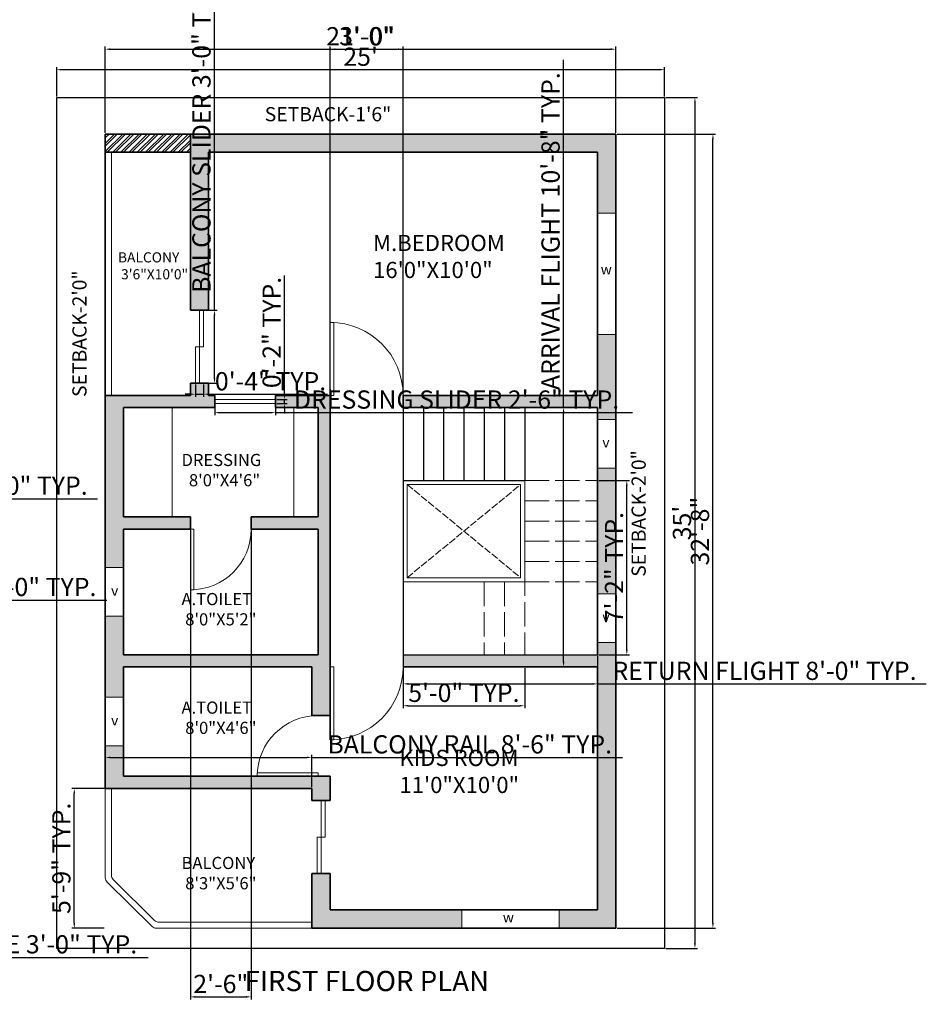
# Model space of a CAD drawing. Units: inches. Extents: x 3488 to 4319, y 780 to 1756.
# Tile 2 of 8: x 3872 to 4319, y 788 to 1274. Entities that reach past the tile are written whole.
import ezdxf

# ---------------------------------------------------------------- set-up
doc = ezdxf.new("R2010")
doc.units = ezdxf.units.IN
doc.linetypes.add('ACAD_ISO02W100', pattern=[15, 12, -3])
for name, color, linetype, lineweight in [('A-ANNO-IDEN', 7, 'Continuous', 13), ('A-ANNO-TEXT', 7, 'Continuous', 18), ('A-ANNO-TITL', 7, 'Continuous', 25), ('A-AREA-IDEN', 7, 'Continuous', 18), ('A-DOOR', 4, 'Continuous', 18), ('A-FLOR-CASE', 32, 'Continuous', 18), ('A-FLOR-OPEN', 3, 'Continuous', 20), ('A-FLOR-OPEN-HIDN', 3, 'ACAD_ISO02W100', 13), ('A-FLOR-RAIL', 7, 'Continuous', 20), ('A-FLOR-STRS', 7, 'Continuous', 25), ('A-FLOR-STRS-OVHD', 8, 'ACAD_ISO02W100', 18), ('A-WALL', 7, 'Continuous', 35), ('A-WALL-PATT', 252, 'Continuous', 13), ('C-PROP', 7, 'Continuous', 25), ('DIM', 9, 'Continuous', 18), ('window', 130, 'Continuous', 18)]:
    doc.layers.add(name, color=color, linetype=linetype, lineweight=lineweight)
doc.styles.get("Standard").update_dxf_attribs({"font": 'arial.ttf'})
doc.dimstyles.new('ISO-25', dxfattribs={"dimtxt": 9, "dimasz": 2.5, "dimexe": 1.25, "dimexo": 0.625, "dimtad": 1, "dimdec": 1, "dimlunit": 3, "dimtxsty": 'Standard', "dimcen": 2.5, "dimclrd": 1, "dimclre": 1, "dimclrt": 1, "dimadec": 0, "dimazin": 0, "dimtfac": 1, "dimtdec": 1, "dimtmove": 0, "dimatfit": 3, "dimfxl": 1, "dimarcsym": 0})

# ---------------------------------------------------------------- blocks, each defined once
blk = doc.blocks.new('*U3')
for p, q in [((0, 0), (0, -6)), ((36, 0), (36, -6))]:
    blk.add_line(p, q)
blk.add_lwpolyline([(0, 0), (0, 36), (1.75, 36), (1.75, 0)], close=True)
blk.add_arc((0, 0), 36, 0, 90)
blk = doc.blocks.new('*D13')
at = {"layer": 'Defpoints', "color": 0, "transparency": 16777216}
for p in [(4189.84, 1249.81), (3889.84, 1236.01), (4189.84, 1236.01)]:
    blk.add_point(p, dxfattribs=at)
at = {"layer": 'DIM', "color": 0, "lineweight": -2, "transparency": 16777216}
for p, q in [((3889.84, 1236.63), (3889.84, 1251.06)), ((3892.34, 1249.81), (4187.34, 1249.81)), ((4189.84, 1236.63), (4189.84, 1251.06))]:
    blk.add_line(p, q, dxfattribs=at)
at = {"layer": 'DIM', "color": 0, "transparency": 16777216}
for points in [[(3892.34, 1250.23), (3892.34, 1249.39), (3889.84, 1249.81)], [(4187.34, 1250.23), (4187.34, 1249.39), (4189.84, 1249.81)]]:
    blk.add_solid(points, dxfattribs=at)
at = {"layer": 'DIM', "color": 0, "transparency": 16777216, "insert": (4039.84, 1255.03), "char_height": 9, "attachment_point": 5}
blk.add_mtext("25'", dxfattribs=at)
blk = doc.blocks.new('*D12')
at = {"layer": 'Defpoints', "color": 0, "transparency": 16777216}
for p in [(4189.84, 1236.01), (4189.84, 816.01), (4204.87, 816.01)]:
    blk.add_point(p, dxfattribs=at)
at = {"layer": 'DIM', "color": 0, "lineweight": -2, "transparency": 16777216}
for p, q in [((4190.47, 1236.01), (4206.12, 1236.01)), ((4204.87, 1233.51), (4204.87, 818.51)), ((4190.47, 816.01), (4206.12, 816.01))]:
    blk.add_line(p, q, dxfattribs=at)
at = {"layer": 'DIM', "color": 0, "transparency": 16777216}
for points in [[(4204.45, 1233.51), (4205.28, 1233.51), (4204.87, 1236.01)], [(4204.45, 818.51), (4205.28, 818.51), (4204.87, 816.01)]]:
    blk.add_solid(points, dxfattribs=at)
at = {"layer": 'DIM', "color": 0, "transparency": 16777216, "insert": (4199.64, 1026.01), "char_height": 9, "attachment_point": 5, "rotation": 90}
blk.add_mtext("35'", dxfattribs=at)
blk = doc.blocks.new('*U9')
for p, q in [((0, 0), (0, 6)), ((36, 0), (36, 6))]:
    blk.add_line(p, q)
blk.add_lwpolyline([(0, 0), (0, -36), (1.75, -36), (1.75, 0)], close=True)
blk.add_arc((0, 0), 36, 270, 0)
blk = doc.blocks.new('*U10')
for p, q in [((0, 0), (0, 6)), ((30, 0), (30, 6))]:
    blk.add_line(p, q)
blk.add_lwpolyline([(0, 0), (0, -30), (1.75, -30), (1.75, 0)], close=True)
blk.add_arc((0, 0), 30, 270, 0)
blk = doc.blocks.new('*U11')
for p, q in [((-30, 0), (-30, 6)), ((0, 0), (0, 6))]:
    blk.add_line(p, q)
blk.add_lwpolyline([(0, 0), (0, -30), (-1.75, -30), (-1.75, 0)], close=True)
blk.add_arc((0, 0), 30, 180, 270)
blk = doc.blocks.new('DOOR-SLIDING-36IN')
for p, q in [((2, 0), (2, 36)), ((4, 18), (4, 36)), ((0, 0), (0, 18)), ((0, 18), (4, 18))]:
    blk.add_line(p, q)
blk = doc.blocks.new('RAIL-BALCONY-CHAMFERED')
for p, q in [((0, 69), (0, 24.92)), ((3, 69), (3, 26.17)), ((23.12, 0.86), (0.89, 22.78)), ((24.35, 3.86), (3.89, 24.04)), ((102, 3), (26.46, 3)), ((102, 0), (25.23, 0))]:
    blk.add_line(p, q)
for centre, start, end in [((3, 24.92), 180, 225.4044), ((6, 26.17), 180, 225.4044), ((25.23, 3), 225.4044, 270), ((26.46, 6), 225.4044, 270)]:
    blk.add_arc(centre, 3, start, end)
blk = doc.blocks.new('STAIR-UPPER-RETURN-BEYOND')
for p, q in [((60, 86), (60, 0)), ((60, 86), (96, 86)), ((60, 76), (96, 76)), ((60, 66), (96, 66)), ((60, 56), (96, 56)), ((60, 46), (96, 46)), ((0, 36), (96, 36)), ((40, 36), (40, 0)), ((50, 36), (50, 0))]:
    blk.add_line(p, q)
blk = doc.blocks.new('STAIR-UPPER-ARRIVAL-FLIGHT')
for p, q in [((0, 128), (0, 0)), ((10, 128), (10, 92)), ((20, 128), (20, 92)), ((30, 128), (30, 92)), ((40, 128), (40, 92)), ((50, 128), (50, 92)), ((60, 128), (60, 92)), ((0, 92), (60, 92))]:
    blk.add_line(p, q)
blk = doc.blocks.new('OPENING-STAIRWELL-FRAME')
for points in [[(60, 50), (0, 50), (0, 0), (60, 0)], [(58, 48), (2, 48), (2, 2), (58, 2)]]:
    blk.add_lwpolyline(points, close=True)
blk = doc.blocks.new('DOOR-SLIDING-30IN')
for p, q in [((30, 2), (0, 2)), ((30, 0), (0, 0))]:
    blk.add_line(p, q)
blk = doc.blocks.new('*D58')
at = {"layer": 'Defpoints', "color": 0, "transparency": 16777216}
for p in [(3962.34, 1131.01), (3967.74, 1131.01), (3962.34, 1095.01)]:
    blk.add_point(p, dxfattribs=at)
at = {"layer": 'DIM', "color": 1, "lineweight": -2, "transparency": 16777216}
for p, q in [((3967.74, 1131.01), (3967.74, 1301.71)), ((3962.97, 1131.01), (3968.99, 1131.01)), ((3967.74, 1097.51), (3967.74, 1128.51)), ((3962.97, 1095.01), (3968.99, 1095.01))]:
    blk.add_line(p, q, dxfattribs=at)
at = {"layer": 'DIM', "color": 1, "transparency": 16777216}
for points in [[(3967.33, 1128.51), (3968.16, 1128.51), (3967.74, 1131.01)], [(3967.33, 1097.51), (3968.16, 1097.51), (3967.74, 1095.01)]]:
    blk.add_solid(points, dxfattribs=at)
at = {"layer": 'DIM', "color": 1, "transparency": 16777216, "insert": (3962.46, 1217.61), "char_height": 9, "attachment_point": 5, "rotation": 90}
blk.add_mtext('BALCONY SLIDER 3\'-0" TYP.', dxfattribs=at)
blk = doc.blocks.new('*D59')
at = {"layer": 'Defpoints', "color": 0, "transparency": 16777216}
for p in [(3958.34, 1095.01), (3962.34, 1095.01), (3962.34, 1089.61)]:
    blk.add_point(p, dxfattribs=at)
at = {"layer": 'DIM', "color": 1, "lineweight": -2, "transparency": 16777216}
for p, q in [((3958.34, 1094.38), (3958.34, 1088.36)), ((3962.34, 1094.38), (3962.34, 1088.36)), ((3955.84, 1089.61), (3953.34, 1089.61)), ((3958.34, 1089.61), (3962.34, 1089.61)), ((3964.84, 1089.61), (4023.45, 1089.61))]:
    blk.add_line(p, q, dxfattribs=at)
at = {"layer": 'DIM', "color": 1, "transparency": 16777216}
for points in [[(3955.84, 1090.02), (3955.84, 1089.19), (3958.34, 1089.61)], [(3964.84, 1090.02), (3964.84, 1089.19), (3962.34, 1089.61)]]:
    blk.add_solid(points, dxfattribs=at)
at = {"layer": 'DIM', "color": 1, "transparency": 16777216, "insert": (3995.4, 1094.83), "char_height": 9, "attachment_point": 5}
blk.add_mtext('0\'-4" TYP.', dxfattribs=at)
blk = doc.blocks.new('*D60')
at = {"layer": 'Defpoints', "color": 0, "transparency": 16777216}
for p in [(3693.99, 997.01), (3753.99, 997.01), (3753.99, 988.01)]:
    blk.add_point(p, dxfattribs=at)
at = {"layer": 'DIM', "color": 1, "lineweight": -2, "transparency": 16777216}
for p, q in [((3693.99, 996.38), (3693.99, 986.76)), ((3753.99, 996.38), (3753.99, 986.76)), ((3696.49, 988.01), (3751.49, 988.01)), ((3753.99, 988.01), (3914.55, 988.01))]:
    blk.add_line(p, q, dxfattribs=at)
at = {"layer": 'DIM', "color": 1, "transparency": 16777216}
for points in [[(3696.49, 988.42), (3696.49, 987.59), (3693.99, 988.01)], [(3751.49, 988.42), (3751.49, 987.59), (3753.99, 988.01)]]:
    blk.add_solid(points, dxfattribs=at)
at = {"layer": 'DIM', "color": 1, "transparency": 16777216, "insert": (3835.52, 993.29), "char_height": 9, "attachment_point": 5}
blk.add_mtext('STAIR OPENING 5\'-0" TYP.', dxfattribs=at)
blk = doc.blocks.new('*D70')
at = {"layer": 'Defpoints', "color": 0, "transparency": 16777216}
for p in [(3756.99, 817.01), (3792.99, 817.01), (3792.99, 811.61)]:
    blk.add_point(p, dxfattribs=at)
at = {"layer": 'DIM', "color": 1, "lineweight": -2, "transparency": 16777216}
for p, q in [((3756.99, 816.38), (3756.99, 810.36)), ((3792.99, 816.38), (3792.99, 810.36)), ((3759.49, 811.61), (3790.49, 811.61)), ((3792.99, 811.61), (3934.96, 811.61))]:
    blk.add_line(p, q, dxfattribs=at)
at = {"layer": 'DIM', "color": 1, "transparency": 16777216}
for points in [[(3759.49, 812.02), (3759.49, 811.19), (3756.99, 811.61)], [(3790.49, 812.02), (3790.49, 811.19), (3792.99, 811.61)]]:
    blk.add_solid(points, dxfattribs=at)
at = {"layer": 'DIM', "color": 1, "transparency": 16777216, "insert": (3865.22, 816.89), "char_height": 9, "attachment_point": 5}
blk.add_mtext('ENTRY GATE 3\'-0" TYP.', dxfattribs=at)
blk = doc.blocks.new('*D72')
at = {"layer": 'Defpoints', "color": 0, "transparency": 16777216}
for p in [(4015.84, 910.31), (3913.84, 895.01), (4015.84, 895.01)]:
    blk.add_point(p, dxfattribs=at)
at = {"layer": 'DIM', "color": 1, "lineweight": -2, "transparency": 16777216}
for p, q in [((3913.84, 895.63), (3913.84, 911.56)), ((3916.34, 910.31), (4013.34, 910.31)), ((4015.84, 895.63), (4015.84, 911.56)), ((4015.84, 910.31), (4169.08, 910.31))]:
    blk.add_line(p, q, dxfattribs=at)
at = {"layer": 'DIM', "color": 1, "transparency": 16777216}
for points in [[(3916.34, 910.72), (3916.34, 909.89), (3913.84, 910.31)], [(4013.34, 910.72), (4013.34, 909.89), (4015.84, 910.31)]]:
    blk.add_solid(points, dxfattribs=at)
at = {"layer": 'DIM', "color": 1, "transparency": 16777216, "insert": (4093.71, 915.59), "char_height": 9, "attachment_point": 5}
blk.add_mtext('BALCONY RAIL 8\'-6" TYP.', dxfattribs=at)
blk = doc.blocks.new('*D73')
at = {"layer": 'Defpoints', "color": 0, "transparency": 16777216}
for p in [(3898.54, 895.01), (3913.84, 895.01), (3913.84, 826.01)]:
    blk.add_point(p, dxfattribs=at)
at = {"layer": 'DIM', "color": 1, "lineweight": -2, "transparency": 16777216}
for p, q in [((3913.22, 895.01), (3897.29, 895.01)), ((3898.54, 828.51), (3898.54, 892.51)), ((3913.22, 826.01), (3897.29, 826.01))]:
    blk.add_line(p, q, dxfattribs=at)
at = {"layer": 'DIM', "color": 1, "transparency": 16777216}
for points in [[(3898.13, 892.51), (3898.96, 892.51), (3898.54, 895.01)], [(3898.13, 828.51), (3898.96, 828.51), (3898.54, 826.01)]]:
    blk.add_solid(points, dxfattribs=at)
at = {"layer": 'DIM', "color": 1, "transparency": 16777216, "insert": (3893.32, 860.51), "char_height": 9, "attachment_point": 5, "rotation": 90}
blk.add_mtext('5\'-9" TYP.', dxfattribs=at)
blk = doc.blocks.new('*D74')
at = {"layer": 'Defpoints', "color": 0, "transparency": 16777216}
for p in [(3693.99, 1047.01), (3753.99, 1047.01), (3753.99, 1038.01)]:
    blk.add_point(p, dxfattribs=at)
at = {"layer": 'DIM', "color": 1, "lineweight": -2, "transparency": 16777216}
for p, q in [((3693.99, 1046.38), (3693.99, 1036.76)), ((3753.99, 1046.38), (3753.99, 1036.76)), ((3696.49, 1038.01), (3751.49, 1038.01)), ((3753.99, 1038.01), (3910, 1038.01))]:
    blk.add_line(p, q, dxfattribs=at)
at = {"layer": 'DIM', "color": 1, "transparency": 16777216}
for points in [[(3696.49, 1038.42), (3696.49, 1037.59), (3693.99, 1038.01)], [(3751.49, 1038.42), (3751.49, 1037.59), (3753.99, 1038.01)]]:
    blk.add_solid(points, dxfattribs=at)
at = {"layer": 'DIM', "color": 1, "transparency": 16777216, "insert": (3833.24, 1043.29), "char_height": 9, "attachment_point": 5}
blk.add_mtext('LOWER FLIGHT 5\'-0" TYP.', dxfattribs=at)
blk = doc.blocks.new('*D78')
at = {"layer": 'Defpoints', "color": 0, "transparency": 16777216}
for p in [(4060.84, 961.01), (4156.84, 961.01), (4156.84, 946.61)]:
    blk.add_point(p, dxfattribs=at)
at = {"layer": 'DIM', "color": 1, "lineweight": -2, "transparency": 16777216}
for p, q in [((4060.84, 960.38), (4060.84, 945.36)), ((4156.84, 960.38), (4156.84, 945.36)), ((4063.34, 946.61), (4154.34, 946.61)), ((4156.84, 946.61), (4319.06, 946.61))]:
    blk.add_line(p, q, dxfattribs=at)
at = {"layer": 'DIM', "color": 1, "transparency": 16777216}
for points in [[(4063.34, 947.02), (4063.34, 946.19), (4060.84, 946.61)], [(4154.34, 947.02), (4154.34, 946.19), (4156.84, 946.61)]]:
    blk.add_solid(points, dxfattribs=at)
at = {"layer": 'DIM', "color": 1, "transparency": 16777216, "insert": (4239.2, 951.89), "char_height": 9, "attachment_point": 5}
blk.add_mtext('RETURN FLIGHT 8\'-0" TYP.', dxfattribs=at)
blk = doc.blocks.new('*D79')
at = {"layer": 'Defpoints', "color": 0, "transparency": 16777216}
for p in [(4156.84, 1047.01), (4171.24, 1047.01), (4156.84, 961.01)]:
    blk.add_point(p, dxfattribs=at)
at = {"layer": 'DIM', "color": 1, "lineweight": -2, "transparency": 16777216}
for p, q in [((4157.47, 1047.01), (4172.49, 1047.01)), ((4171.24, 963.51), (4171.24, 1044.51)), ((4157.47, 961.01), (4172.49, 961.01))]:
    blk.add_line(p, q, dxfattribs=at)
at = {"layer": 'DIM', "color": 1, "transparency": 16777216}
for points in [[(4170.83, 1044.51), (4171.66, 1044.51), (4171.24, 1047.01)], [(4170.83, 963.51), (4171.66, 963.51), (4171.24, 961.01)]]:
    blk.add_solid(points, dxfattribs=at)
at = {"layer": 'DIM', "color": 1, "transparency": 16777216, "insert": (4166.1, 1004.01), "char_height": 9, "attachment_point": 5, "rotation": 90}
blk.add_mtext('7\'-2" TYP.', dxfattribs=at)
blk = doc.blocks.new('*D80')
at = {"layer": 'Defpoints', "color": 0, "transparency": 16777216}
for p in [(4120.84, 1083.01), (4140.04, 1083.01), (4120.84, 955.01)]:
    blk.add_point(p, dxfattribs=at)
at = {"layer": 'DIM', "color": 1, "lineweight": -2, "transparency": 16777216}
for p, q in [((4140.04, 1083.01), (4140.04, 1254.63)), ((4121.47, 1083.01), (4141.29, 1083.01)), ((4140.04, 957.51), (4140.04, 1080.51)), ((4121.47, 955.01), (4141.29, 955.01))]:
    blk.add_line(p, q, dxfattribs=at)
at = {"layer": 'DIM', "color": 1, "transparency": 16777216}
for points in [[(4139.63, 1080.51), (4140.46, 1080.51), (4140.04, 1083.01)], [(4139.63, 957.51), (4140.46, 957.51), (4140.04, 955.01)]]:
    blk.add_solid(points, dxfattribs=at)
at = {"layer": 'DIM', "color": 1, "transparency": 16777216, "insert": (4134.77, 1170.07), "char_height": 9, "attachment_point": 5, "rotation": 90}
blk.add_mtext('ARRIVAL FLIGHT 10\'-8" TYP.', dxfattribs=at)
blk = doc.blocks.new('*D81')
at = {"layer": 'Defpoints', "color": 0, "transparency": 16777216}
for p in [(4060.84, 955.01), (4120.84, 955.01), (4120.84, 935.81)]:
    blk.add_point(p, dxfattribs=at)
at = {"layer": 'DIM', "color": 1, "lineweight": -2, "transparency": 16777216}
for p, q in [((4060.84, 954.38), (4060.84, 934.56)), ((4120.84, 954.38), (4120.84, 934.56)), ((4063.34, 935.81), (4118.34, 935.81))]:
    blk.add_line(p, q, dxfattribs=at)
at = {"layer": 'DIM', "color": 1, "transparency": 16777216}
for points in [[(4063.34, 936.22), (4063.34, 935.39), (4060.84, 935.81)], [(4118.34, 936.22), (4118.34, 935.39), (4120.84, 935.81)]]:
    blk.add_solid(points, dxfattribs=at)
at = {"layer": 'DIM', "color": 1, "transparency": 16777216, "insert": (4090.84, 941.03), "char_height": 9, "attachment_point": 5}
blk.add_mtext('5\'-0" TYP.', dxfattribs=at)
blk = doc.blocks.new('*D82')
at = {"layer": 'Defpoints', "color": 0, "transparency": 16777216}
for p in [(3967.84, 1085.01), (3997.84, 1085.01), (3997.84, 1080.51)]:
    blk.add_point(p, dxfattribs=at)
at = {"layer": 'DIM', "color": 1, "lineweight": -2, "transparency": 16777216}
for p, q in [((3967.84, 1084.38), (3967.84, 1079.26)), ((3997.84, 1084.38), (3997.84, 1079.26)), ((3970.34, 1080.51), (3995.34, 1080.51)), ((3997.84, 1080.51), (4174.08, 1080.51))]:
    blk.add_line(p, q, dxfattribs=at)
at = {"layer": 'DIM', "color": 1, "transparency": 16777216}
for points in [[(3970.34, 1080.92), (3970.34, 1080.09), (3967.84, 1080.51)], [(3995.34, 1080.92), (3995.34, 1080.09), (3997.84, 1080.51)]]:
    blk.add_solid(points, dxfattribs=at)
at = {"layer": 'DIM', "color": 1, "transparency": 16777216, "insert": (4087.21, 1085.79), "char_height": 9, "attachment_point": 5}
blk.add_mtext('DRESSING SLIDER 2\'-6" TYP.', dxfattribs=at)
blk = doc.blocks.new('*D83')
at = {"layer": 'Defpoints', "color": 0, "transparency": 16777216}
for p in [(3997.84, 1087.01), (3997.84, 1085.01), (4002.34, 1087.01)]:
    blk.add_point(p, dxfattribs=at)
at = {"layer": 'DIM', "color": 1, "lineweight": -2, "transparency": 16777216}
for p, q in [((4002.34, 1089.51), (4002.34, 1148.12)), ((3998.47, 1087.01), (4003.59, 1087.01)), ((3998.47, 1085.01), (4003.59, 1085.01)), ((4002.34, 1085.01), (4002.34, 1087.01)), ((4002.34, 1082.51), (4002.34, 1080.01))]:
    blk.add_line(p, q, dxfattribs=at)
at = {"layer": 'DIM', "color": 1, "transparency": 16777216}
for points in [[(4001.93, 1089.51), (4002.76, 1089.51), (4002.34, 1087.01)], [(4001.93, 1082.51), (4002.76, 1082.51), (4002.34, 1085.01)]]:
    blk.add_solid(points, dxfattribs=at)
at = {"layer": 'DIM', "color": 1, "transparency": 16777216, "insert": (3997.12, 1120.06), "char_height": 9, "attachment_point": 5, "rotation": 90}
blk.add_mtext('0\'-2" TYP.', dxfattribs=at)
blk = doc.blocks.new('*D110')
at = {"layer": 'Defpoints', "color": 0, "transparency": 16777216}
for p in [(4165.84, 1259.91), (3913.84, 1218.01), (4165.84, 1218.01)]:
    blk.add_point(p, dxfattribs=at)
at = {"layer": 'DIM', "color": 1, "lineweight": -2, "transparency": 16777216}
for p, q in [((3913.84, 1218.63), (3913.84, 1261.16)), ((3916.34, 1259.91), (4163.34, 1259.91)), ((4165.84, 1218.63), (4165.84, 1261.16))]:
    blk.add_line(p, q, dxfattribs=at)
at = {"layer": 'DIM', "color": 1, "transparency": 16777216}
for points in [[(3916.34, 1260.32), (3916.34, 1259.49), (3913.84, 1259.91)], [(4163.34, 1260.32), (4163.34, 1259.49), (4165.84, 1259.91)]]:
    blk.add_solid(points, dxfattribs=at)
at = {"layer": 'DIM', "color": 1, "transparency": 16777216, "insert": (4039.84, 1265.13), "char_height": 9, "attachment_point": 5}
blk.add_mtext('21\'-0"', dxfattribs=at)
blk = doc.blocks.new('*D111')
at = {"layer": 'Defpoints', "color": 0, "transparency": 16777216}
for p in [(4165.84, 1218.01), (4213.74, 1218.01), (4165.84, 826.01)]:
    blk.add_point(p, dxfattribs=at)
at = {"layer": 'DIM', "color": 1, "lineweight": -2, "transparency": 16777216}
for p, q in [((4166.47, 1218.01), (4214.99, 1218.01)), ((4213.74, 828.51), (4213.74, 1215.51)), ((4166.47, 826.01), (4214.99, 826.01))]:
    blk.add_line(p, q, dxfattribs=at)
at = {"layer": 'DIM', "color": 1, "transparency": 16777216}
for points in [[(4213.33, 1215.51), (4214.16, 1215.51), (4213.74, 1218.01)], [(4213.33, 828.51), (4214.16, 828.51), (4213.74, 826.01)]]:
    blk.add_solid(points, dxfattribs=at)
at = {"layer": 'DIM', "color": 1, "transparency": 16777216, "insert": (4208.52, 1022.01), "char_height": 9, "attachment_point": 5, "rotation": 90}
blk.add_mtext('32\'-8"', dxfattribs=at)
blk = doc.blocks.new('*D119')
at = {"layer": 'Defpoints', "color": 0, "transparency": 16777216}
for p in [(4060.84, 1259.91), (4024.84, 1089.01), (4060.84, 1089.01)]:
    blk.add_point(p, dxfattribs=at)
at = {"layer": 'DIM', "color": 1, "lineweight": -2, "transparency": 16777216}
for p, q in [((4024.84, 1089.63), (4024.84, 1261.16)), ((4027.34, 1259.91), (4058.34, 1259.91)), ((4060.84, 1089.63), (4060.84, 1261.16))]:
    blk.add_line(p, q, dxfattribs=at)
at = {"layer": 'DIM', "color": 1, "transparency": 16777216}
for points in [[(4027.34, 1260.32), (4027.34, 1259.49), (4024.84, 1259.91)], [(4058.34, 1260.32), (4058.34, 1259.49), (4060.84, 1259.91)]]:
    blk.add_solid(points, dxfattribs=at)
at = {"layer": 'DIM', "color": 1, "transparency": 16777216, "insert": (4042.84, 1265.13), "char_height": 9, "attachment_point": 5}
blk.add_mtext('3\'-0"', dxfattribs=at)
blk = doc.blocks.new('*D120')
at = {"layer": 'Defpoints', "color": 0, "transparency": 16777216}
for p in [(3955.84, 1023.01), (3985.84, 1023.01), (3985.84, 792.11)]:
    blk.add_point(p, dxfattribs=at)
at = {"layer": 'DIM', "color": 1, "lineweight": -2, "transparency": 16777216}
for p, q in [((3955.84, 1022.38), (3955.84, 790.86)), ((3985.84, 1022.38), (3985.84, 790.86)), ((3958.34, 792.11), (3983.34, 792.11))]:
    blk.add_line(p, q, dxfattribs=at)
at = {"layer": 'DIM', "color": 1, "transparency": 16777216}
for points in [[(3958.34, 792.52), (3958.34, 791.69), (3955.84, 792.11)], [(3983.34, 792.52), (3983.34, 791.69), (3985.84, 792.11)]]:
    blk.add_solid(points, dxfattribs=at)
at = {"layer": 'DIM', "color": 1, "transparency": 16777216, "insert": (3970.84, 797.33), "char_height": 9, "attachment_point": 5}
blk.add_mtext('2\'-6"', dxfattribs=at)

msp = doc.modelspace()

# ---------------------------------------------------------------- hatches: boundary and pattern name
at = {"layer": 'A-WALL-PATT'}
h = msp.add_hatch(color=256, dxfattribs=at)
h.dxf.hatch_style = 1
h.paths.add_polyline_path([(4156.84, 1209.01), (4156.84, 1179.01), (4165.84, 1179.01), (4165.84, 1218.01), (3955.84, 1218.01), (3955.84, 1131.01), (3964.84, 1131.01), (3964.84, 1209.01)])
h.paths.add_polyline_path([(3913.84, 1004.01), (3922.84, 1004.01), (3922.84, 1023.01), (3955.84, 1023.01), (3955.84, 1029.01), (3922.84, 1029.01), (3922.84, 1083.01), (3967.84, 1083.01), (3967.84, 1089.01), (3964.84, 1089.01), (3964.84, 1095.01), (3955.84, 1095.01), (3955.84, 1089.01), (3913.84, 1089.01)])
h.paths.add_polyline_path([(3913.84, 940.01), (3922.84, 940.01), (3922.84, 955.01), (4015.84, 955.01), (4015.84, 931.01), (4024.84, 931.01), (4024.84, 1011.01), (4024.84, 1083.01), (4024.84, 1089.01), (3997.84, 1089.01), (3997.84, 1083.01), (4018.84, 1083.01), (4018.84, 1029.01), (3985.84, 1029.01), (3985.84, 1023.01), (4018.84, 1023.01), (4018.84, 961.01), (3922.84, 961.01), (3922.84, 980.01), (3913.84, 980.01)])
h.paths.add_polyline_path([(3922.84, 916.01), (3913.84, 916.01), (3913.84, 895.01), (4015.84, 895.01), (4015.84, 889.01), (4024.84, 889.01), (4024.84, 901.01), (4018.84, 901.01), (3988.84, 901.01), (3922.84, 901.01)])
h.paths.add_polyline_path([(4024.84, 853.01), (4015.84, 853.01), (4015.84, 826.01), (4089.84, 826.01), (4089.84, 835.01), (4024.84, 835.01)])
h.paths.add_polyline_path([(4137.84, 835.01), (4137.84, 826.01), (4165.84, 826.01), (4165.84, 966.98), (4156.84, 966.98), (4156.84, 961.01), (4060.84, 961.01), (4060.84, 955.01), (4156.84, 955.01), (4156.84, 835.01)])
h.paths.add_polyline_path([(4156.84, 990.98), (4165.84, 990.98), (4165.84, 1053.04), (4156.84, 1053.04)])
h.paths.add_polyline_path([(4156.84, 1089.01), (4060.84, 1089.01), (4060.84, 1083.01), (4156.84, 1083.01), (4156.84, 1077.04), (4165.84, 1077.04), (4165.84, 1119.01), (4156.84, 1119.01)])
h.paths.add_polyline_path([(3918.33, 1143.47), (3954.99, 1143.47), (3954.99, 1162.13), (3918.33, 1162.13)], flags=9)
h = msp.add_hatch(dxfattribs=at)
h.set_pattern_fill('ANSI32', color=256, scale=0.3)
h.set_pattern_definition([(45, (0, -1100.1302), (-2.0205576, 2.0205576), []), (45, (1.347, -1100.1302), (-2.0205576, 2.0205576), [])])
h.paths.add_polyline_path([(3913.84, 1218.01), (3913.84, 1209.01), (3955.84, 1209.01), (3955.84, 1218.01)])

# ---------------------------------------------------------------- linework, layer by layer
at = {"layer": 'A-FLOR-CASE'}
for p, q in [((3946.84, 1029.01), (3946.84, 1083.01)), ((4006.84, 1083.01), (4006.84, 1029.01))]:
    msp.add_line(p, q, dxfattribs=at)
at = {"layer": 'A-FLOR-OPEN-HIDN', "ltscale": 0.3}
for p, q in [((4062.84, 1045.01), (4118.84, 999.01)), ((4062.84, 999.01), (4118.84, 1045.01))]:
    msp.add_line(p, q, dxfattribs=at)
at = {"layer": 'A-FLOR-RAIL'}
msp.add_line((3916.84, 1089.01), (3916.84, 1209.01), dxfattribs=at)
at = {"layer": 'A-FLOR-STRS'}
msp.add_line((4060.84, 961.01), (4156.84, 961.01), dxfattribs=at)
at = {"layer": 'A-WALL'}
for p, q in [((3913.84, 1218.01), (4165.84, 1218.01)), ((3913.84, 895.01), (3913.84, 1218.01)), ((3955.84, 1218.01), (3955.84, 1131.01)), ((4165.84, 1218.01), (4165.84, 826.01)), ((3913.84, 1209.01), (3955.84, 1209.01)), ((3964.84, 1209.01), (3964.84, 1131.01)), ((3964.84, 1209.01), (4156.84, 1209.01)), ((4156.84, 1209.01), (4156.84, 1089.01)), ((3955.84, 1131.01), (3964.84, 1131.01)), ((3955.84, 1095.01), (3964.84, 1095.01)), ((3955.84, 1095.01), (3955.84, 1089.01)), ((3964.84, 1095.01), (3964.84, 1089.01)), ((3913.84, 1089.01), (3955.84, 1089.01)), ((3964.84, 1089.01), (3967.84, 1089.01)), ((3967.84, 1089.01), (3967.84, 1083.01)), ((3997.84, 1089.01), (4024.84, 1089.01)), ((3997.84, 1089.01), (3997.84, 1083.01)), ((4024.84, 1083.01), (4024.84, 1092.01)), ((4060.84, 1089.01), (4156.84, 1089.01)), ((4060.84, 1089.01), (4060.84, 1083.01)), ((3922.84, 1083.01), (3967.84, 1083.01)), ((3922.84, 1029.01), (3922.84, 1083.01)), ((3997.84, 1083.01), (4018.84, 1083.01)), ((4018.84, 1083.01), (4018.84, 1029.01)), ((4024.84, 1083.01), (4024.84, 955.01)), ((4060.84, 1083.01), (4156.84, 1083.01)), ((4156.84, 1083.01), (4156.84, 961.01)), ((3922.84, 1029.01), (3955.84, 1029.01)), ((3955.84, 1029.01), (3955.84, 1023.01)), ((3985.84, 1029.01), (4018.84, 1029.01)), ((3985.84, 1029.01), (3985.84, 1023.01)), ((3922.84, 1023.01), (3955.84, 1023.01)), ((3922.84, 961.01), (3922.84, 1023.01)), ((3985.84, 1023.01), (4018.84, 1023.01)), ((4018.84, 1023.01), (4018.84, 961.01)), ((4024.84, 1011.01), (4024.84, 919.01)), ((3922.84, 961.01), (4018.84, 961.01)), ((3922.84, 955.01), (4015.84, 955.01)), ((3922.84, 901.01), (3922.84, 955.01)), ((4015.84, 955.01), (4015.84, 931.01)), ((4060.84, 955.01), (4156.84, 955.01)), ((4156.84, 955.01), (4156.84, 835.01)), ((4015.84, 931.01), (4024.84, 931.01)), ((3922.84, 901.01), (4024.84, 901.01)), ((4024.84, 901.01), (4024.84, 889.01)), ((3913.84, 895.01), (4015.84, 895.01)), ((4015.84, 895.01), (4015.84, 889.01)), ((4015.84, 889.01), (4024.84, 889.01)), ((4015.84, 853.01), (4015.84, 826.01)), ((4015.84, 853.01), (4024.84, 853.01)), ((4024.84, 853.01), (4024.84, 835.01)), ((4024.84, 835.01), (4156.84, 835.01)), ((4015.84, 826.01), (4165.84, 826.01))]:
    msp.add_line(p, q, dxfattribs=at)
at = {"layer": 'C-PROP'}
for p, q in [((3889.84, 1236.01), (4189.84, 1236.01)), ((3889.84, 816.01), (3889.84, 1236.01)), ((4189.84, 1236.01), (4189.84, 816.01)), ((4189.84, 816.01), (3889.84, 816.01))]:
    msp.add_line(p, q, dxfattribs=at)
at = {"layer": 'window'}
for p, q in [((4156.84, 1179.01), (4165.84, 1179.01)), ((4156.84, 1119.01), (4165.84, 1119.01)), ((4156.84, 1077.04), (4165.84, 1077.04)), ((4156.84, 1053.04), (4165.84, 1053.04)), ((3922.84, 1004.01), (3913.84, 1004.01)), ((4156.84, 990.98), (4165.84, 990.98)), ((3922.84, 980.01), (3913.84, 980.01)), ((4156.84, 966.98), (4165.84, 966.98)), ((3922.84, 940.01), (3913.84, 940.01)), ((3922.84, 916.01), (3913.84, 916.01)), ((4089.84, 835.01), (4089.84, 826.01)), ((4137.84, 835.01), (4137.84, 826.01))]:
    msp.add_line(p, q, dxfattribs=at)

# ---------------------------------------------------------------- block references
at = {"layer": 'A-DOOR'}
for name, p in [('DOOR-SLIDING-36IN', (3958.34, 1095.01)), ('*U3', (4024.84, 1089.01)), ('DOOR-SLIDING-30IN', (3967.84, 1085.01)), ('*U10', (3955.84, 1023.01)), ('*U9', (4024.84, 955.01)), ('DOOR-SLIDING-36IN', (4018.34, 853.01))]:
    msp.add_blockref(name, p, dxfattribs=at)
at = {"layer": 'A-DOOR', "rotation": 270}
msp.add_blockref('*U11', (4018.84, 901.01), dxfattribs=at)
at = {"layer": 'A-FLOR-OPEN'}
msp.add_blockref('OPENING-STAIRWELL-FRAME', (4060.85, 997.01), dxfattribs=at)
at = {"layer": 'A-FLOR-RAIL'}
msp.add_blockref('RAIL-BALCONY-CHAMFERED', (3913.84, 826.01), dxfattribs=at)
at = {"layer": 'A-FLOR-STRS'}
msp.add_blockref('STAIR-UPPER-ARRIVAL-FLIGHT', (4060.84, 955.01), dxfattribs=at)
at = {"layer": 'A-FLOR-STRS-OVHD'}
msp.add_blockref('STAIR-UPPER-RETURN-BEYOND', (4060.84, 961.01), dxfattribs=at)

# ---------------------------------------------------------------- texts
at = {"layer": 'A-ANNO-IDEN'}
for s, p in [('w', (4158.36, 1148.73)), ('v', (4159.18, 1063.32)), ('v', (3916.7, 990.1)), ('v', (4159.18, 977.07)), ('v', (3916.7, 926.1)), ('w', (4110.06, 828.84))]:
    msp.add_text(s, height=5, dxfattribs=at).set_placement(p)
at = {"layer": 'A-ANNO-TEXT', "insert": (3992.52, 1231.32), "char_height": 7, "attachment_point": 1}
msp.add_mtext_dynamic_manual_height_columns('\\pxt7;{SETBACK-1\'6"}', width=83.4163, gutter_width=25, heights=[0], dxfattribs=at)
at = {"layer": 'A-ANNO-TEXT', "char_height": 7, "attachment_point": 1, "rotation": 90}
for insert in [(3897.59, 1088.23), (4173.59, 999.48)]:
    msp.add_mtext_dynamic_manual_height_columns('\\pxt7;{SETBACK-2\'0"}', width=83.4163, gutter_width=25, heights=[0], dxfattribs=dict(at, insert=insert))
at = {"layer": 'A-ANNO-TITL', "insert": (3982.59, 804.94), "char_height": 10, "attachment_point": 1}
msp.add_mtext_dynamic_manual_height_columns('FIRST FLOOR PLAN', width=202.5735, gutter_width=25, heights=[0], dxfattribs=at)
at = {"layer": 'A-AREA-IDEN', "attachment_point": 1}
for s, insert, char_height in [('M.BEDROOM\\P16\'0"X10\'0"', (4046.01, 1168.26), 8), ('BALCONY\\P 3\'6"X10\'0"', (3920.09, 1159.65), 5), ('DRESSING\\P  8\'0"X4\'6"', (3951.46, 1060.14), 6), ('A.TOILET\\P 8\'0"X5\'2"', (3951.46, 991.47), 6), ('A.TOILET\\P 8\'0"X4\'6"', (3951.46, 937.9), 6), ('KIDS ROOM\\P11\'0"X10\'0"', (4059.05, 914.06), 8), ('BALCONY\\P 8\'3"X5\'6"', (3951.46, 861.2), 6)]:
    msp.add_mtext_dynamic_manual_height_columns(s, width=83.4163, gutter_width=25, heights=[0], dxfattribs=dict(at, insert=insert, char_height=char_height))

# ---------------------------------------------------------------- dimensions: what is measured, and where the dimension line sits
at = {"layer": 'DIM'}
for base, p1, p2, text, picture, middle in [((3967.74, 1131.01), (3962.34, 1095.01), (3962.34, 1131.01), 'BALCONY SLIDER <> TYP.', '*D58', (3962.46, 1217.61)), ((4140.04, 1083.01), (4120.84, 955.01), (4120.84, 1083.01), 'ARRIVAL FLIGHT <> TYP.', '*D80', (4134.77, 1170.07)), ((4002.34, 1087.01), (3997.84, 1085.01), (3997.84, 1087.01), '<> TYP.', '*D83', (3997.12, 1120.06)), ((4171.24, 1047.01), (4156.84, 961.01), (4156.84, 1047.01), '<> TYP.', '*D79', (4166.1, 1004.01)), ((3898.54, 895.01), (3913.84, 826.01), (3913.84, 895.01), '<> TYP.', '*D73', (3893.32, 860.51))]:
    dim = msp.add_linear_dim(base=base, p1=p1, p2=p2, angle=90, text=text, dimstyle='ISO-25', override={"dimdec": 1, "dimlfac": 1, "dimrnd": 0, "dimzin": 1, "dimdsep": 46, "dimlunit": 4, "dimfrac": 2}, dxfattribs=at)
    dim.commit()
    dim.dimension.update_dxf_attribs({"geometry": picture, "text_midpoint": middle})
for base, p1, p2, override, picture, middle in [((4165.84, 1259.91), (3913.84, 1218.01), (4165.84, 1218.01), {"dimdec": 1, "dimlfac": 1, "dimrnd": 0, "dimzin": 1, "dimdsep": 46, "dimlunit": 4, "dimfrac": 2}, '*D110', (4039.84, 1265.13)), ((4060.84, 1259.91), (4024.84, 1089.01), (4060.84, 1089.01), {"dimdec": 1, "dimlfac": 1, "dimrnd": 0, "dimzin": 1, "dimdsep": 46, "dimlunit": 4, "dimfrac": 2}, '*D119', (4042.84, 1265.13)), ((4189.84, 1249.81), (3889.84, 1236.01), (4189.84, 1236.01), {"dimclrd": 0, "dimclre": 0, "dimclrt": 0}, '*D13', (4039.84, 1255.03)), ((3985.84, 792.11), (3955.84, 1023.01), (3985.84, 1023.01), {"dimdec": 1, "dimlfac": 1, "dimrnd": 0, "dimzin": 1, "dimdsep": 46, "dimlunit": 4, "dimfrac": 2}, '*D120', (3970.84, 797.33))]:
    dim = msp.add_linear_dim(base=base, p1=p1, p2=p2, dimstyle='ISO-25', override=override, dxfattribs=at)
    dim.commit()
    dim.dimension.update_dxf_attribs({"geometry": picture, "text_midpoint": middle})
for base, p1, p2, override, picture, middle in [((4204.87, 816.01), (4189.84, 1236.01), (4189.84, 816.01), {"dimclrd": 0, "dimclre": 0, "dimclrt": 0}, '*D12', (4199.64, 1026.01)), ((4213.74, 1218.01), (4165.84, 826.01), (4165.84, 1218.01), {"dimdec": 1, "dimlfac": 1, "dimrnd": 0, "dimzin": 1, "dimdsep": 46, "dimlunit": 4, "dimfrac": 2}, '*D111', (4208.52, 1022.01))]:
    dim = msp.add_linear_dim(base=base, p1=p1, p2=p2, angle=90, dimstyle='ISO-25', override=override, dxfattribs=at)
    dim.commit()
    dim.dimension.update_dxf_attribs({"geometry": picture, "text_midpoint": middle})
for base, p1, p2, text, picture, middle in [((3997.84, 1080.51), (3967.84, 1085.01), (3997.84, 1085.01), 'DRESSING SLIDER <> TYP.', '*D82', (4087.21, 1085.79)), ((3962.34, 1089.61), (3958.34, 1095.01), (3962.34, 1095.01), '<> TYP.', '*D59', (3995.4, 1094.83)), ((3753.99, 1038.01), (3693.99, 1047.01), (3753.99, 1047.01), 'LOWER FLIGHT <> TYP.', '*D74', (3833.24, 1043.29)), ((3753.99, 988.01), (3693.99, 997.01), (3753.99, 997.01), 'STAIR OPENING <> TYP.', '*D60', (3835.52, 993.29)), ((4156.84, 946.61), (4060.84, 961.01), (4156.84, 961.01), 'RETURN FLIGHT <> TYP.', '*D78', (4239.2, 951.89)), ((4120.84, 935.81), (4060.84, 955.01), (4120.84, 955.01), '<> TYP.', '*D81', (4090.84, 941.03)), ((4015.84, 910.31), (3913.84, 895.01), (4015.84, 895.01), 'BALCONY RAIL <> TYP.', '*D72', (4093.71, 915.59)), ((3792.99, 811.61), (3756.99, 817.01), (3792.99, 817.01), 'ENTRY GATE <> TYP.', '*D70', (3865.22, 816.89))]:
    dim = msp.add_linear_dim(base=base, p1=p1, p2=p2, text=text, dimstyle='ISO-25', override={"dimdec": 1, "dimlfac": 1, "dimrnd": 0, "dimzin": 1, "dimdsep": 46, "dimlunit": 4, "dimfrac": 2}, dxfattribs=at)
    dim.commit()
    dim.dimension.update_dxf_attribs({"geometry": picture, "text_midpoint": middle})

doc.saveas('drawing.dxf')
